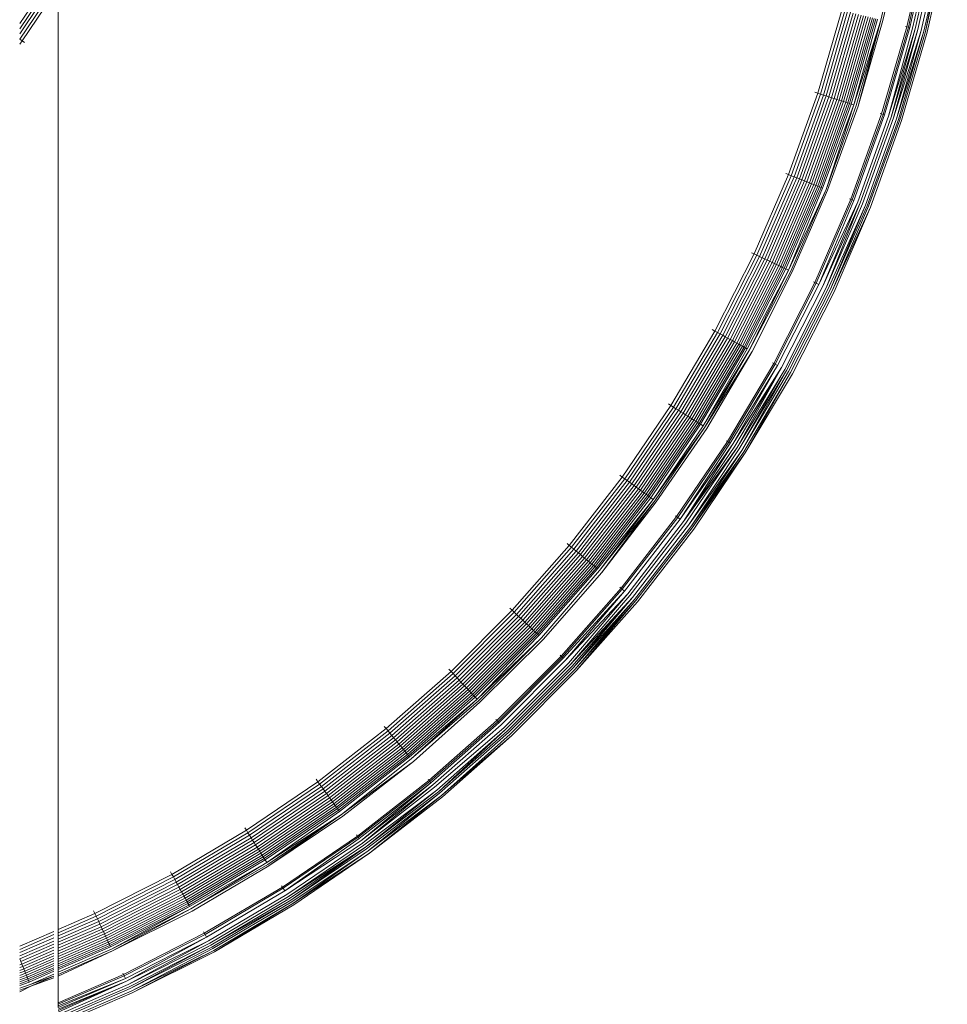
# Model space of a CAD drawing. Units: inches. Extents: x 64 to 1167, y 117 to 939.
# Tile 48 of 56: x 1130.6487 to 1131.3636, y 499.9133 to 500.6716. Entities that reach past the tile are written whole.
import ezdxf

# ---------------------------------------------------------------- set-up
doc = ezdxf.new("R2010")
doc.units = ezdxf.units.IN
doc.header["$MEASUREMENT"] = 0
doc.layers.add('A-FLOR-FIXT', color=8, linetype='Continuous', lineweight=18)

msp = doc.modelspace()

# ---------------------------------------------------------------- linework, layer by layer
at = {"layer": 'A-FLOR-FIXT'}
for p, q in [((1131.3125, 500.67123), (1131.32746, 500.73815)), ((1131.31402, 500.67084), (1131.329, 500.73786)), ((1131.33251, 500.66609), (1131.34775, 500.73428)), ((1131.33362, 500.6658), (1131.34888, 500.73407)), ((1131.33472, 500.66552), (1131.35, 500.73385)), ((1131.33688, 500.66497), (1131.35219, 500.73344)), ((1131.33895, 500.66444), (1131.35428, 500.73304)), ((1131.34088, 500.66394), (1131.35625, 500.73266)), ((1131.34347, 500.66327), (1131.35887, 500.73216)), ((1131.3456, 500.66273), (1131.36103, 500.73175)), ((1131.34672, 500.66244), (1131.36103, 500.73175)), ((1131.34672, 500.66244), (1131.36216, 500.73153)), ((1131.34815, 500.66207), (1131.36362, 500.73126)), ((1130.67845, 500.69852), (1130.67845, 499.97088)), ((1130.64872, 500.66854), (1130.66031, 500.68559)), ((1130.64872, 500.66461), (1130.66217, 500.6844)), ((1130.64872, 500.66061), (1130.66407, 500.6832)), ((1130.64881, 500.6567), (1130.666, 500.68198)), ((1130.65067, 500.65534), (1130.66794, 500.68075)), ((1131.26378, 500.61498), (1131.28237, 500.67896)), ((1131.26596, 500.61427), (1131.28459, 500.67839)), ((1131.26813, 500.61357), (1131.2868, 500.67783)), ((1131.27027, 500.61288), (1131.28898, 500.67727)), ((1131.27237, 500.61219), (1131.29112, 500.67672)), ((1131.27443, 500.61152), (1131.29321, 500.67618)), ((1131.27643, 500.61087), (1131.29525, 500.67566)), ((1131.27837, 500.61024), (1131.29722, 500.67515)), ((1131.28023, 500.60964), (1131.29912, 500.67466)), ((1131.28202, 500.60906), (1131.30094, 500.67419)), ((1131.28371, 500.60851), (1131.30267, 500.67375)), ((1131.28532, 500.60799), (1131.3043, 500.67333)), ((1131.28682, 500.6075), (1131.30583, 500.67294)), ((1131.28821, 500.60705), (1131.30725, 500.67257)), ((1131.28949, 500.60663), (1131.30855, 500.67224)), ((1131.29169, 500.60592), (1131.30973, 500.67194)), ((1131.29169, 500.60592), (1131.3125, 500.67123)), ((1131.29337, 500.60537), (1131.3125, 500.67123)), ((1131.29486, 500.60489), (1131.3125, 500.67123)), ((1131.29486, 500.60489), (1131.31402, 500.67084)), ((1131.31301, 500.59899), (1131.33251, 500.66609)), ((1131.3141, 500.59863), (1131.33362, 500.6658)), ((1131.31519, 500.59828), (1131.33472, 500.66552)), ((1131.33139, 500.66638), (1131.33251, 500.66609)), ((1131.33251, 500.66609), (1131.33362, 500.6658)), ((1131.33362, 500.6658), (1131.33472, 500.66552)), ((1131.31834, 500.59726), (1131.33688, 500.66497)), ((1131.31834, 500.59726), (1131.33895, 500.66444)), ((1131.32031, 500.59662), (1131.33895, 500.66444)), ((1131.32031, 500.59662), (1131.34088, 500.66394)), ((1131.32213, 500.59602), (1131.34088, 500.66394)), ((1131.32213, 500.59602), (1131.34347, 500.66327)), ((1131.32453, 500.59524), (1131.34347, 500.66327)), ((1131.32453, 500.59524), (1131.3456, 500.66273)), ((1131.32587, 500.59481), (1131.3456, 500.66273)), ((1131.32697, 500.59445), (1131.34672, 500.66244)), ((1131.32837, 500.594), (1131.34815, 500.66207)), ((1130.64872, 500.65283), (1130.65067, 500.65534)), ((1130.65067, 500.65534), (1130.64881, 500.6567)), ((1130.65254, 500.65399), (1130.65067, 500.65534)), ((1131.24121, 500.5523), (1131.26378, 500.61498)), ((1131.24335, 500.55145), (1131.26596, 500.61427)), ((1131.24547, 500.55061), (1131.26813, 500.61357)), ((1131.24756, 500.54979), (1131.27027, 500.61288)), ((1131.24961, 500.54897), (1131.27237, 500.61219)), ((1131.26158, 500.6157), (1131.26378, 500.61498)), ((1131.26378, 500.61498), (1131.26596, 500.61427)), ((1131.26596, 500.61427), (1131.26813, 500.61357)), ((1131.26813, 500.61357), (1131.27027, 500.61288)), ((1131.27027, 500.61288), (1131.27237, 500.61219)), ((1131.27237, 500.61219), (1131.27443, 500.61152)), ((1131.25162, 500.54818), (1131.27443, 500.61152)), ((1131.25358, 500.5474), (1131.27643, 500.61087)), ((1131.25547, 500.54665), (1131.27837, 500.61024)), ((1131.25729, 500.54593), (1131.28023, 500.60964)), ((1131.25904, 500.54524), (1131.28202, 500.60906)), ((1131.2607, 500.54458), (1131.28371, 500.60851)), ((1131.26227, 500.54396), (1131.28532, 500.60799)), ((1131.26374, 500.54338), (1131.28682, 500.6075)), ((1131.2651, 500.54284), (1131.28821, 500.60705)), ((1131.26635, 500.54235), (1131.28949, 500.60663)), ((1131.26748, 500.5419), (1131.29169, 500.60592)), ((1131.27014, 500.54085), (1131.29169, 500.60592)), ((1131.27014, 500.54085), (1131.29337, 500.60537)), ((1131.27125, 500.54041), (1131.29486, 500.60489)), ((1131.27443, 500.61152), (1131.27643, 500.61087)), ((1131.27643, 500.61087), (1131.27837, 500.61024)), ((1131.27837, 500.61024), (1131.28023, 500.60964)), ((1131.28023, 500.60964), (1131.28202, 500.60906)), ((1131.28202, 500.60906), (1131.28371, 500.60851)), ((1131.28371, 500.60851), (1131.28532, 500.60799)), ((1131.28532, 500.60799), (1131.28682, 500.6075)), ((1131.28682, 500.6075), (1131.28821, 500.60705)), ((1131.28821, 500.60705), (1131.28949, 500.60663)), ((1131.28949, 500.60663), (1131.29169, 500.60592)), ((1131.28934, 500.53324), (1131.31301, 500.59899)), ((1131.29041, 500.53282), (1131.3141, 500.59863)), ((1131.29147, 500.5324), (1131.31519, 500.59828)), ((1131.29455, 500.53118), (1131.31834, 500.59726)), ((1131.31301, 500.59899), (1131.31191, 500.59934)), ((1131.3141, 500.59863), (1131.31301, 500.59899)), ((1131.31519, 500.59828), (1131.3141, 500.59863)), ((1131.29647, 500.53042), (1131.32031, 500.59662)), ((1131.29826, 500.52971), (1131.32213, 500.59602)), ((1131.3006, 500.52878), (1131.32453, 500.59524)), ((1131.30191, 500.52827), (1131.32587, 500.59481)), ((1131.30298, 500.52784), (1131.32697, 500.59445)), ((1131.30436, 500.5273), (1131.32837, 500.594)), ((1131.21475, 500.49115), (1131.24121, 500.5523)), ((1131.21683, 500.49018), (1131.24335, 500.55145)), ((1131.23906, 500.55315), (1131.24121, 500.5523)), ((1131.24121, 500.5523), (1131.24335, 500.55145)), ((1131.24335, 500.55145), (1131.24547, 500.55061)), ((1131.21889, 500.48921), (1131.24547, 500.55061)), ((1131.22093, 500.48825), (1131.24756, 500.54979)), ((1131.22293, 500.48731), (1131.24961, 500.54897)), ((1131.22488, 500.48639), (1131.25162, 500.54818)), ((1131.22679, 500.48549), (1131.25358, 500.5474)), ((1131.22863, 500.48462), (1131.25547, 500.54665)), ((1131.2304, 500.48379), (1131.25729, 500.54593)), ((1131.2321, 500.48299), (1131.25904, 500.54524)), ((1131.23372, 500.48223), (1131.2607, 500.54458)), ((1131.23524, 500.48151), (1131.26227, 500.54396)), ((1131.24547, 500.55061), (1131.24756, 500.54979)), ((1131.24756, 500.54979), (1131.24961, 500.54897)), ((1131.24961, 500.54897), (1131.25162, 500.54818)), ((1131.25162, 500.54818), (1131.25358, 500.5474)), ((1131.25358, 500.5474), (1131.25547, 500.54665)), ((1131.25547, 500.54665), (1131.25729, 500.54593)), ((1131.25729, 500.54593), (1131.25904, 500.54524)), ((1131.25904, 500.54524), (1131.2607, 500.54458)), ((1131.2607, 500.54458), (1131.26227, 500.54396)), ((1131.26227, 500.54396), (1131.26374, 500.54338)), ((1131.23667, 500.48084), (1131.26374, 500.54338)), ((1131.238, 500.48022), (1131.2651, 500.54284)), ((1131.23921, 500.47964), (1131.26635, 500.54235)), ((1131.2413, 500.47866), (1131.26748, 500.5419)), ((1131.2413, 500.47866), (1131.27014, 500.54085)), ((1131.2429, 500.47791), (1131.27014, 500.54085)), ((1131.24398, 500.4774), (1131.27125, 500.54041)), ((1131.26374, 500.54338), (1131.2651, 500.54284)), ((1131.2651, 500.54284), (1131.26635, 500.54235)), ((1131.26635, 500.54235), (1131.26748, 500.5419)), ((1131.26159, 500.46911), (1131.28934, 500.53324)), ((1131.26263, 500.46862), (1131.29041, 500.53282)), ((1131.26468, 500.46766), (1131.29147, 500.5324)), ((1131.26468, 500.46766), (1131.29455, 500.53118)), ((1131.26761, 500.46628), (1131.29455, 500.53118)), ((1131.26761, 500.46628), (1131.29647, 500.53042)), ((1131.27027, 500.46503), (1131.29647, 500.53042)), ((1131.27027, 500.46503), (1131.29826, 500.52971)), ((1131.27184, 500.46429), (1131.3006, 500.52878)), ((1131.27321, 500.46364), (1131.3006, 500.52878)), ((1131.28827, 500.53367), (1131.28934, 500.53324)), ((1131.28934, 500.53324), (1131.29041, 500.53282)), ((1131.29041, 500.53282), (1131.29147, 500.5324)), ((1131.27321, 500.46364), (1131.30191, 500.52827)), ((1131.27487, 500.46287), (1131.30298, 500.52784)), ((1131.27487, 500.46287), (1131.30436, 500.5273)), ((1131.27651, 500.46209), (1131.30436, 500.5273)), ((1131.1845, 500.43179), (1131.21475, 500.49115)), ((1131.21266, 500.49214), (1131.21475, 500.49115)), ((1131.21475, 500.49115), (1131.21683, 500.49018)), ((1131.18652, 500.43068), (1131.21683, 500.49018)), ((1131.18851, 500.42959), (1131.21889, 500.48921)), ((1131.19049, 500.4285), (1131.22093, 500.48825)), ((1131.19242, 500.42744), (1131.22293, 500.48731)), ((1131.19432, 500.4264), (1131.22488, 500.48639)), ((1131.19616, 500.42538), (1131.22679, 500.48549)), ((1131.19794, 500.4244), (1131.22863, 500.48462)), ((1131.19966, 500.42346), (1131.2304, 500.48379)), ((1131.21683, 500.49018), (1131.21889, 500.48921)), ((1131.21889, 500.48921), (1131.22093, 500.48825)), ((1131.22093, 500.48825), (1131.22293, 500.48731)), ((1131.22293, 500.48731), (1131.22488, 500.48639)), ((1131.22488, 500.48639), (1131.22679, 500.48549)), ((1131.22679, 500.48549), (1131.22863, 500.48462)), ((1131.22863, 500.48462), (1131.2304, 500.48379)), ((1131.2304, 500.48379), (1131.2321, 500.48299)), ((1131.20131, 500.42255), (1131.2321, 500.48299)), ((1131.20287, 500.42169), (1131.23372, 500.48223)), ((1131.20435, 500.42088), (1131.23524, 500.48151)), ((1131.20573, 500.42012), (1131.23667, 500.48084)), ((1131.20702, 500.41941), (1131.238, 500.48022)), ((1131.2082, 500.41877), (1131.23921, 500.47964)), ((1131.20926, 500.41818), (1131.2413, 500.47866)), ((1131.21105, 500.4172), (1131.2413, 500.47866)), ((1131.21105, 500.4172), (1131.2429, 500.47791)), ((1131.21334, 500.41594), (1131.24398, 500.4774)), ((1131.2321, 500.48299), (1131.23372, 500.48223)), ((1131.23372, 500.48223), (1131.23524, 500.48151)), ((1131.23524, 500.48151), (1131.23667, 500.48084)), ((1131.23667, 500.48084), (1131.238, 500.48022)), ((1131.238, 500.48022), (1131.23921, 500.47964)), ((1131.23921, 500.47964), (1131.2413, 500.47866)), ((1131.22987, 500.40685), (1131.26159, 500.46911)), ((1131.23087, 500.4063), (1131.26263, 500.46862)), ((1131.26055, 500.4696), (1131.26159, 500.46911)), ((1131.26159, 500.46911), (1131.26263, 500.46862)), ((1131.26263, 500.46862), (1131.26468, 500.46766)), ((1131.23286, 500.40521), (1131.26468, 500.46766)), ((1131.2357, 500.40365), (1131.26761, 500.46628)), ((1131.23827, 500.40223), (1131.27027, 500.46503)), ((1131.23979, 500.4014), (1131.27184, 500.46429)), ((1131.24112, 500.40066), (1131.27321, 500.46364)), ((1131.24272, 500.39978), (1131.27487, 500.46287)), ((1131.24432, 500.39891), (1131.27651, 500.46209)), ((1131.15059, 500.37445), (1131.1845, 500.43179)), ((1131.15253, 500.37321), (1131.18652, 500.43068)), ((1131.1845, 500.43179), (1131.18248, 500.4329)), ((1131.18652, 500.43068), (1131.1845, 500.43179)), ((1131.18851, 500.42959), (1131.18652, 500.43068)), ((1131.15445, 500.37199), (1131.18851, 500.42959)), ((1131.15635, 500.37079), (1131.19049, 500.4285)), ((1131.15822, 500.3696), (1131.19242, 500.42744)), ((1131.16004, 500.36845), (1131.19432, 500.4264)), ((1131.16182, 500.36732), (1131.19616, 500.42538)), ((1131.16354, 500.36623), (1131.19794, 500.4244)), ((1131.1652, 500.36518), (1131.19966, 500.42346)), ((1131.16678, 500.36417), (1131.20131, 500.42255)), ((1131.19049, 500.4285), (1131.18851, 500.42959)), ((1131.19242, 500.42744), (1131.19049, 500.4285)), ((1131.19432, 500.4264), (1131.19242, 500.42744)), ((1131.19616, 500.42538), (1131.19432, 500.4264)), ((1131.19794, 500.4244), (1131.19616, 500.42538)), ((1131.19966, 500.42346), (1131.19794, 500.4244)), ((1131.20131, 500.42255), (1131.19966, 500.42346)), ((1131.20287, 500.42169), (1131.20131, 500.42255)), ((1131.16829, 500.36321), (1131.20287, 500.42169)), ((1131.16971, 500.36231), (1131.20435, 500.42088)), ((1131.17104, 500.36146), (1131.20573, 500.42012)), ((1131.17228, 500.36068), (1131.20702, 500.41941)), ((1131.17342, 500.35996), (1131.2082, 500.41877)), ((1131.17537, 500.35872), (1131.20926, 500.41818)), ((1131.17537, 500.35872), (1131.21105, 500.4172)), ((1131.17686, 500.35778), (1131.21105, 500.4172)), ((1131.17686, 500.35778), (1131.21334, 500.41594)), ((1131.17837, 500.35681), (1131.21334, 500.41594)), ((1131.20435, 500.42088), (1131.20287, 500.42169)), ((1131.20573, 500.42012), (1131.20435, 500.42088)), ((1131.20702, 500.41941), (1131.20573, 500.42012)), ((1131.2082, 500.41877), (1131.20702, 500.41941)), ((1131.20926, 500.41818), (1131.2082, 500.41877)), ((1131.22987, 500.40685), (1131.22886, 500.40741)), ((1131.1943, 500.34671), (1131.22987, 500.40685)), ((1131.19527, 500.34609), (1131.23087, 500.4063)), ((1131.19623, 500.34548), (1131.23286, 500.40521)), ((1131.19811, 500.34429), (1131.23286, 500.40521)), ((1131.19811, 500.34429), (1131.2357, 500.40365)), ((1131.19991, 500.34314), (1131.2357, 500.40365)), ((1131.2016, 500.34207), (1131.2357, 500.40365)), ((1131.2016, 500.34207), (1131.23827, 500.40223)), ((1131.20315, 500.34109), (1131.23827, 500.40223)), ((1131.20315, 500.34109), (1131.23979, 500.4014)), ((1131.20514, 500.33982), (1131.23979, 500.4014)), ((1131.20514, 500.33982), (1131.24112, 500.40066)), ((1131.20669, 500.33885), (1131.24272, 500.39978)), ((1131.20794, 500.33805), (1131.24272, 500.39978)), ((1131.23087, 500.4063), (1131.22987, 500.40685)), ((1131.23286, 500.40521), (1131.23087, 500.4063)), ((1131.20794, 500.33805), (1131.24432, 500.39891)), ((1131.11314, 500.31934), (1131.15059, 500.37445)), ((1131.115, 500.31799), (1131.15253, 500.37321)), ((1131.11684, 500.31665), (1131.15445, 500.37199)), ((1131.11866, 500.31533), (1131.15635, 500.37079)), ((1131.12045, 500.31403), (1131.15822, 500.3696)), ((1131.14864, 500.37568), (1131.15059, 500.37445)), ((1131.15059, 500.37445), (1131.15253, 500.37321)), ((1131.15253, 500.37321), (1131.15445, 500.37199)), ((1131.15445, 500.37199), (1131.15635, 500.37079)), ((1131.15635, 500.37079), (1131.15822, 500.3696)), ((1131.15822, 500.3696), (1131.16004, 500.36845)), ((1131.1222, 500.31276), (1131.16004, 500.36845)), ((1131.1239, 500.31152), (1131.16182, 500.36732)), ((1131.12555, 500.31033), (1131.16354, 500.36623)), ((1131.12714, 500.30917), (1131.1652, 500.36518)), ((1131.12865, 500.30807), (1131.16678, 500.36417)), ((1131.1301, 500.30702), (1131.16829, 500.36321)), ((1131.13146, 500.30603), (1131.16971, 500.36231)), ((1131.16004, 500.36845), (1131.16182, 500.36732)), ((1131.16182, 500.36732), (1131.16354, 500.36623)), ((1131.16354, 500.36623), (1131.1652, 500.36518)), ((1131.1652, 500.36518), (1131.16678, 500.36417)), ((1131.16678, 500.36417), (1131.16829, 500.36321)), ((1131.16829, 500.36321), (1131.16971, 500.36231)), ((1131.16971, 500.36231), (1131.17104, 500.36146)), ((1131.13274, 500.3051), (1131.17104, 500.36146)), ((1131.13393, 500.30424), (1131.17228, 500.36068)), ((1131.13501, 500.30345), (1131.17342, 500.35996)), ((1131.13688, 500.30209), (1131.17537, 500.35872)), ((1131.13688, 500.30209), (1131.17686, 500.35778)), ((1131.13831, 500.30105), (1131.17686, 500.35778)), ((1131.13928, 500.30035), (1131.17837, 500.35681)), ((1131.17104, 500.36146), (1131.17228, 500.36068)), ((1131.17228, 500.36068), (1131.17342, 500.35996)), ((1131.17342, 500.35996), (1131.17537, 500.35872)), ((1131.15502, 500.28891), (1131.1943, 500.34671)), ((1131.19332, 500.34733), (1131.1943, 500.34671)), ((1131.1943, 500.34671), (1131.19527, 500.34609)), ((1131.15595, 500.28824), (1131.19527, 500.34609)), ((1131.15778, 500.28691), (1131.19623, 500.34548)), ((1131.15778, 500.28691), (1131.19811, 500.34429)), ((1131.1604, 500.285), (1131.19811, 500.34429)), ((1131.1604, 500.285), (1131.19991, 500.34314)), ((1131.1604, 500.285), (1131.2016, 500.34207)), ((1131.16202, 500.28383), (1131.2016, 500.34207)), ((1131.16418, 500.28226), (1131.20315, 500.34109)), ((1131.16418, 500.28226), (1131.20514, 500.33982)), ((1131.16596, 500.28097), (1131.20514, 500.33982)), ((1131.19527, 500.34609), (1131.19623, 500.34548)), ((1131.16596, 500.28097), (1131.20669, 500.33885)), ((1131.16689, 500.28029), (1131.20669, 500.33885)), ((1131.16689, 500.28029), (1131.20794, 500.33805)), ((1131.16824, 500.27931), (1131.20794, 500.33805)), ((1131.07231, 500.2667), (1131.11314, 500.31934)), ((1131.07408, 500.26523), (1131.115, 500.31799)), ((1131.07583, 500.26378), (1131.11684, 500.31665)), ((1131.11127, 500.3207), (1131.11314, 500.31934)), ((1131.11314, 500.31934), (1131.115, 500.31799)), ((1131.115, 500.31799), (1131.11684, 500.31665)), ((1131.11684, 500.31665), (1131.11866, 500.31533)), ((1131.07757, 500.26235), (1131.11866, 500.31533)), ((1131.07927, 500.26094), (1131.12045, 500.31403)), ((1131.08093, 500.25956), (1131.1222, 500.31276)), ((1131.08256, 500.25822), (1131.1239, 500.31152)), ((1131.08412, 500.25692), (1131.12555, 500.31033)), ((1131.08564, 500.25567), (1131.12714, 500.30917)), ((1131.11866, 500.31533), (1131.12045, 500.31403)), ((1131.12045, 500.31403), (1131.1222, 500.31276)), ((1131.1222, 500.31276), (1131.1239, 500.31152)), ((1131.1239, 500.31152), (1131.12555, 500.31033)), ((1131.12555, 500.31033), (1131.12714, 500.30917)), ((1131.12714, 500.30917), (1131.12865, 500.30807)), ((1131.08708, 500.25447), (1131.12865, 500.30807)), ((1131.08846, 500.25334), (1131.1301, 500.30702)), ((1131.08976, 500.25226), (1131.13146, 500.30603)), ((1131.09097, 500.25126), (1131.13274, 500.3051)), ((1131.0921, 500.25032), (1131.13393, 500.30424)), ((1131.09314, 500.24946), (1131.13501, 500.30345)), ((1131.09408, 500.24869), (1131.13688, 500.30209)), ((1131.09565, 500.24739), (1131.13688, 500.30209)), ((1131.12865, 500.30807), (1131.1301, 500.30702)), ((1131.1301, 500.30702), (1131.13146, 500.30603)), ((1131.13146, 500.30603), (1131.13274, 500.3051)), ((1131.13274, 500.3051), (1131.13393, 500.30424)), ((1131.13393, 500.30424), (1131.13501, 500.30345)), ((1131.13501, 500.30345), (1131.13688, 500.30209)), ((1131.09565, 500.24739), (1131.13831, 500.30105)), ((1131.09749, 500.24587), (1131.13831, 500.30105)), ((1131.09749, 500.24587), (1131.13928, 500.30035)), ((1131.11219, 500.2337), (1131.15502, 500.28891)), ((1131.11308, 500.23297), (1131.15595, 500.28824)), ((1131.11482, 500.23152), (1131.15778, 500.28691)), ((1131.15502, 500.28891), (1131.15409, 500.28959)), ((1131.15595, 500.28824), (1131.15502, 500.28891)), ((1131.15778, 500.28691), (1131.15595, 500.28824)), ((1131.11732, 500.22946), (1131.1604, 500.285)), ((1131.11886, 500.22819), (1131.16202, 500.28383)), ((1131.12092, 500.22648), (1131.16418, 500.28226)), ((1131.12261, 500.22508), (1131.16596, 500.28097)), ((1131.1235, 500.22435), (1131.16689, 500.28029)), ((1131.12478, 500.22328), (1131.16824, 500.27931)), ((1131.02825, 500.21672), (1131.07231, 500.2667)), ((1131.02992, 500.21515), (1131.07408, 500.26523)), ((1131.03158, 500.21359), (1131.07583, 500.26378)), ((1131.07053, 500.26817), (1131.07231, 500.2667)), ((1131.07231, 500.2667), (1131.07408, 500.26523)), ((1131.07408, 500.26523), (1131.07583, 500.26378)), ((1131.07583, 500.26378), (1131.07757, 500.26235)), ((1131.03322, 500.21205), (1131.07757, 500.26235)), ((1131.03483, 500.21054), (1131.07927, 500.26094)), ((1131.03641, 500.20906), (1131.08093, 500.25956)), ((1131.03794, 500.20762), (1131.08256, 500.25822)), ((1131.03943, 500.20622), (1131.08412, 500.25692)), ((1131.07757, 500.26235), (1131.07927, 500.26094)), ((1131.07927, 500.26094), (1131.08093, 500.25956)), ((1131.08093, 500.25956), (1131.08256, 500.25822)), ((1131.08256, 500.25822), (1131.08412, 500.25692)), ((1131.08412, 500.25692), (1131.08564, 500.25567)), ((1131.04086, 500.20488), (1131.08564, 500.25567)), ((1131.04223, 500.2036), (1131.08708, 500.25447)), ((1131.04353, 500.20237), (1131.08846, 500.25334)), ((1131.04476, 500.20122), (1131.08976, 500.25226)), ((1131.04591, 500.20014), (1131.09097, 500.25126)), ((1131.04697, 500.19914), (1131.0921, 500.25032)), ((1131.04796, 500.19821), (1131.09314, 500.24946)), ((1131.04884, 500.19738), (1131.09408, 500.24869)), ((1131.08564, 500.25567), (1131.08708, 500.25447)), ((1131.08708, 500.25447), (1131.08846, 500.25334)), ((1131.08846, 500.25334), (1131.08976, 500.25226)), ((1131.08976, 500.25226), (1131.09097, 500.25126)), ((1131.09097, 500.25126), (1131.0921, 500.25032)), ((1131.0921, 500.25032), (1131.09314, 500.24946)), ((1131.09314, 500.24946), (1131.09408, 500.24869)), ((1131.05093, 500.19543), (1131.09565, 500.24739)), ((1131.05224, 500.19419), (1131.09749, 500.24587)), ((1131.06598, 500.18129), (1131.11219, 500.2337)), ((1131.06682, 500.1805), (1131.11308, 500.23297)), ((1131.11219, 500.2337), (1131.1113, 500.23444)), ((1131.11308, 500.23297), (1131.11219, 500.2337)), ((1131.11482, 500.23152), (1131.11308, 500.23297)), ((1131.06765, 500.17972), (1131.11482, 500.23152)), ((1131.06928, 500.17819), (1131.11482, 500.23152)), ((1131.06928, 500.17819), (1131.11732, 500.22946)), ((1131.07157, 500.17604), (1131.11732, 500.22946)), ((1131.07297, 500.17472), (1131.11886, 500.22819)), ((1131.07297, 500.17472), (1131.12092, 500.22648)), ((1131.07424, 500.17353), (1131.12092, 500.22648)), ((1131.07535, 500.17249), (1131.12092, 500.22648)), ((1131.02656, 500.2183), (1131.02825, 500.21672)), ((1131.07535, 500.17249), (1131.12261, 500.22508)), ((1131.07668, 500.17124), (1131.12261, 500.22508)), ((1131.07668, 500.17124), (1131.1235, 500.22435)), ((1131.07776, 500.17023), (1131.1235, 500.22435)), ((1131.07776, 500.17023), (1131.12478, 500.22328)), ((1130.98114, 500.16961), (1131.02825, 500.21672)), ((1130.98271, 500.16794), (1131.02992, 500.21515)), ((1130.98427, 500.16628), (1131.03158, 500.21359)), ((1130.98581, 500.16464), (1131.03322, 500.21205)), ((1130.98732, 500.16302), (1131.03483, 500.21054)), ((1131.02825, 500.21672), (1131.02992, 500.21515)), ((1131.02992, 500.21515), (1131.03158, 500.21359)), ((1131.03158, 500.21359), (1131.03322, 500.21205)), ((1131.03322, 500.21205), (1131.03483, 500.21054)), ((1131.03483, 500.21054), (1131.03641, 500.20906)), ((1130.9888, 500.16145), (1131.03641, 500.20906)), ((1130.99024, 500.15992), (1131.03794, 500.20762)), ((1130.99164, 500.15843), (1131.03943, 500.20622)), ((1130.99298, 500.157), (1131.04086, 500.20488)), ((1130.99426, 500.15563), (1131.04223, 500.2036)), ((1131.03641, 500.20906), (1131.03794, 500.20762)), ((1131.03794, 500.20762), (1131.03943, 500.20622)), ((1131.03943, 500.20622), (1131.04086, 500.20488)), ((1131.04086, 500.20488), (1131.04223, 500.2036)), ((1131.04223, 500.2036), (1131.04353, 500.20237)), ((1130.99549, 500.15433), (1131.04353, 500.20237)), ((1130.99664, 500.1531), (1131.04476, 500.20122)), ((1130.99772, 500.15195), (1131.04591, 500.20014)), ((1130.99872, 500.15088), (1131.04697, 500.19914)), ((1130.99964, 500.1499), (1131.04796, 500.19821)), ((1131.00122, 500.14822), (1131.04884, 500.19738)), ((1131.00122, 500.14822), (1131.05093, 500.19543)), ((1131.00243, 500.14693), (1131.05093, 500.19543)), ((1131.04353, 500.20237), (1131.04476, 500.20122)), ((1131.04476, 500.20122), (1131.04591, 500.20014)), ((1131.04591, 500.20014), (1131.04697, 500.19914)), ((1131.04697, 500.19914), (1131.04796, 500.19821)), ((1131.04796, 500.19821), (1131.04884, 500.19738)), ((1131.00325, 500.14606), (1131.05224, 500.19419)), ((1131.01657, 500.13188), (1131.06598, 500.18129)), ((1131.01736, 500.13104), (1131.06682, 500.1805)), ((1131.06514, 500.18208), (1131.06598, 500.18129)), ((1131.06598, 500.18129), (1131.06682, 500.1805)), ((1131.06682, 500.1805), (1131.06765, 500.17972)), ((1131.01814, 500.13021), (1131.06765, 500.17972)), ((1131.01967, 500.12858), (1131.06928, 500.17819)), ((1131.02182, 500.12628), (1131.07157, 500.17604)), ((1131.02314, 500.12489), (1131.07297, 500.17472)), ((1131.02432, 500.12362), (1131.07424, 500.17353)), ((1131.02537, 500.12251), (1131.07535, 500.17249)), ((1130.93116, 500.12555), (1130.98114, 500.16961)), ((1130.93263, 500.12378), (1130.98271, 500.16794)), ((1130.93408, 500.12203), (1130.98427, 500.16628)), ((1130.97956, 500.17129), (1130.98114, 500.16961)), ((1130.98114, 500.16961), (1130.98271, 500.16794)), ((1130.98271, 500.16794), (1130.98427, 500.16628)), ((1130.98427, 500.16628), (1130.98581, 500.16464)), ((1131.02662, 500.12118), (1131.07668, 500.17124)), ((1131.02763, 500.1201), (1131.07776, 500.17023)), ((1130.93551, 500.12029), (1130.98581, 500.16464)), ((1130.93692, 500.11859), (1130.98732, 500.16302)), ((1130.9383, 500.11692), (1130.9888, 500.16145)), ((1130.93964, 500.1153), (1130.99024, 500.15992)), ((1130.94094, 500.11373), (1130.99164, 500.15843)), ((1130.98581, 500.16464), (1130.98732, 500.16302)), ((1130.98732, 500.16302), (1130.9888, 500.16145)), ((1130.9888, 500.16145), (1130.99024, 500.15992)), ((1130.99024, 500.15992), (1130.99164, 500.15843)), ((1130.99164, 500.15843), (1130.99298, 500.157)), ((1130.94219, 500.11222), (1130.99298, 500.157)), ((1130.94338, 500.11078), (1130.99426, 500.15563)), ((1130.94452, 500.1094), (1130.99549, 500.15433)), ((1130.9456, 500.1081), (1130.99664, 500.1531)), ((1130.9466, 500.10689), (1130.99772, 500.15195)), ((1130.94754, 500.10576), (1130.99872, 500.15088)), ((1130.94839, 500.10472), (1130.99964, 500.1499)), ((1130.99298, 500.157), (1130.99426, 500.15563)), ((1130.99426, 500.15563), (1130.99549, 500.15433)), ((1130.99549, 500.15433), (1130.99664, 500.1531)), ((1130.99664, 500.1531), (1130.99772, 500.15195)), ((1130.99772, 500.15195), (1130.99872, 500.15088)), ((1130.99872, 500.15088), (1130.99964, 500.1499)), ((1130.99964, 500.1499), (1131.00122, 500.14822)), ((1130.94917, 500.10378), (1131.00122, 500.14822)), ((1130.95047, 500.10221), (1131.00122, 500.14822)), ((1130.95047, 500.10221), (1131.00243, 500.14693)), ((1130.95214, 500.1002), (1131.00325, 500.14606)), ((1130.92969, 500.12733), (1130.93116, 500.12555)), ((1130.96416, 500.08567), (1131.01657, 500.13188)), ((1130.96489, 500.08478), (1131.01736, 500.13104)), ((1130.96562, 500.0839), (1131.01814, 500.13021)), ((1130.96704, 500.08218), (1131.01967, 500.12858)), ((1131.01578, 500.13272), (1131.01657, 500.13188)), ((1131.01657, 500.13188), (1131.01736, 500.13104)), ((1131.01736, 500.13104), (1131.01814, 500.13021)), ((1130.87852, 500.08472), (1130.93116, 500.12555)), ((1130.87987, 500.08286), (1130.93263, 500.12378)), ((1130.88121, 500.08101), (1130.93408, 500.12203)), ((1130.88253, 500.0792), (1130.93551, 500.12029)), ((1130.93116, 500.12555), (1130.93263, 500.12378)), ((1130.93263, 500.12378), (1130.93408, 500.12203)), ((1130.93408, 500.12203), (1130.93551, 500.12029)), ((1130.93551, 500.12029), (1130.93692, 500.11859)), ((1130.9684, 500.08054), (1131.02182, 500.12628)), ((1130.97027, 500.07828), (1131.02314, 500.12489)), ((1130.97138, 500.07694), (1131.02314, 500.12489)), ((1130.97138, 500.07694), (1131.02432, 500.12362)), ((1130.97235, 500.07577), (1131.02537, 500.12251)), ((1130.97381, 500.07399), (1131.02662, 500.12118)), ((1130.97381, 500.07399), (1131.02763, 500.1201)), ((1130.97465, 500.07299), (1131.02763, 500.1201)), ((1130.88383, 500.07741), (1130.93692, 500.11859)), ((1130.8851, 500.07566), (1130.9383, 500.11692)), ((1130.88634, 500.07396), (1130.93964, 500.1153)), ((1130.88753, 500.07231), (1130.94094, 500.11373)), ((1130.88869, 500.07072), (1130.94219, 500.11222)), ((1130.93692, 500.11859), (1130.9383, 500.11692)), ((1130.9383, 500.11692), (1130.93964, 500.1153)), ((1130.93964, 500.1153), (1130.94094, 500.11373)), ((1130.94094, 500.11373), (1130.94219, 500.11222)), ((1130.94219, 500.11222), (1130.94338, 500.11078)), ((1130.88979, 500.0692), (1130.94338, 500.11078)), ((1130.89084, 500.06776), (1130.94452, 500.1094)), ((1130.89183, 500.0664), (1130.9456, 500.1081)), ((1130.89276, 500.06512), (1130.9466, 500.10689)), ((1130.89362, 500.06393), (1130.94754, 500.10576)), ((1130.89441, 500.06284), (1130.94839, 500.10472)), ((1130.94338, 500.11078), (1130.94452, 500.1094)), ((1130.94452, 500.1094), (1130.9456, 500.1081)), ((1130.9456, 500.1081), (1130.9466, 500.10689)), ((1130.9466, 500.10689), (1130.94754, 500.10576)), ((1130.94754, 500.10576), (1130.94839, 500.10472)), ((1130.94839, 500.10472), (1130.94917, 500.10378)), ((1130.89513, 500.06186), (1130.94917, 500.10378)), ((1130.8968, 500.05955), (1130.95047, 500.10221)), ((1130.8968, 500.05955), (1130.95214, 500.1002)), ((1130.89786, 500.05809), (1130.95214, 500.1002)), ((1130.82341, 500.04727), (1130.87852, 500.08472)), ((1130.82465, 500.04533), (1130.87987, 500.08286)), ((1130.87852, 500.08472), (1130.87716, 500.08659)), ((1130.87987, 500.08286), (1130.87852, 500.08472)), ((1130.88121, 500.08101), (1130.87987, 500.08286)), ((1130.90894, 500.04284), (1130.96416, 500.08567)), ((1130.90962, 500.04191), (1130.96489, 500.08478)), ((1130.91029, 500.04099), (1130.96562, 500.0839)), ((1130.9116, 500.03918), (1130.96562, 500.0839)), ((1130.9116, 500.03918), (1130.96704, 500.08218)), ((1130.91285, 500.03746), (1130.96704, 500.08218)), ((1130.96342, 500.08655), (1130.96416, 500.08567)), ((1130.96416, 500.08567), (1130.96489, 500.08478)), ((1130.96489, 500.08478), (1130.96562, 500.0839)), ((1130.82587, 500.0434), (1130.88121, 500.08101)), ((1130.82707, 500.04151), (1130.88253, 500.0792)), ((1130.82826, 500.03964), (1130.88383, 500.07741)), ((1130.82941, 500.03781), (1130.8851, 500.07566)), ((1130.83054, 500.03604), (1130.88634, 500.07396)), ((1130.88253, 500.0792), (1130.88121, 500.08101)), ((1130.88383, 500.07741), (1130.88253, 500.0792)), ((1130.8851, 500.07566), (1130.88383, 500.07741)), ((1130.88634, 500.07396), (1130.8851, 500.07566)), ((1130.88753, 500.07231), (1130.88634, 500.07396)), ((1130.91285, 500.03746), (1130.9684, 500.08054)), ((1130.91403, 500.03584), (1130.97027, 500.07828)), ((1130.91511, 500.03436), (1130.97027, 500.07828)), ((1130.91511, 500.03436), (1130.97138, 500.07694)), ((1130.91606, 500.03304), (1130.97235, 500.07577)), ((1130.91725, 500.03141), (1130.97235, 500.07577)), ((1130.91725, 500.03141), (1130.97381, 500.07399)), ((1130.91844, 500.02977), (1130.97381, 500.07399)), ((1130.83163, 500.03432), (1130.88753, 500.07231)), ((1130.83268, 500.03266), (1130.88869, 500.07072)), ((1130.83369, 500.03108), (1130.88979, 500.0692)), ((1130.83465, 500.02957), (1130.89084, 500.06776)), ((1130.83555, 500.02815), (1130.89183, 500.0664)), ((1130.88869, 500.07072), (1130.88753, 500.07231)), ((1130.88979, 500.0692), (1130.88869, 500.07072)), ((1130.89084, 500.06776), (1130.88979, 500.0692)), ((1130.89183, 500.0664), (1130.89084, 500.06776)), ((1130.89276, 500.06512), (1130.89183, 500.0664)), ((1130.91844, 500.02977), (1130.97465, 500.07299)), ((1130.83639, 500.02681), (1130.89276, 500.06512)), ((1130.83718, 500.02558), (1130.89362, 500.06393)), ((1130.8379, 500.02444), (1130.89441, 500.06284)), ((1130.83914, 500.02249), (1130.89513, 500.06186)), ((1130.83914, 500.02249), (1130.8968, 500.05955)), ((1130.84008, 500.021), (1130.8968, 500.05955)), ((1130.84072, 500.01999), (1130.8968, 500.05955)), ((1130.89362, 500.06393), (1130.89276, 500.06512)), ((1130.89441, 500.06284), (1130.89362, 500.06393)), ((1130.89513, 500.06186), (1130.89441, 500.06284)), ((1130.84072, 500.01999), (1130.89786, 500.05809)), ((1130.76607, 500.01335), (1130.82341, 500.04727)), ((1130.76717, 500.01134), (1130.82465, 500.04533)), ((1130.76827, 500.00934), (1130.82587, 500.0434)), ((1130.82218, 500.04922), (1130.82341, 500.04727)), ((1130.82341, 500.04727), (1130.82465, 500.04533)), ((1130.82465, 500.04533), (1130.82587, 500.0434)), ((1130.82587, 500.0434), (1130.82707, 500.04151)), ((1130.90827, 500.04377), (1130.90894, 500.04284)), ((1130.76936, 500.00737), (1130.82707, 500.04151)), ((1130.77042, 500.00544), (1130.82826, 500.03964)), ((1130.77146, 500.00354), (1130.82941, 500.03781)), ((1130.77248, 500.0017), (1130.83054, 500.03604)), ((1130.82707, 500.04151), (1130.82826, 500.03964)), ((1130.82826, 500.03964), (1130.82941, 500.03781)), ((1130.82941, 500.03781), (1130.83054, 500.03604)), ((1130.83054, 500.03604), (1130.83163, 500.03432)), ((1130.85115, 500.00356), (1130.90894, 500.04284)), ((1130.85177, 500.00259), (1130.90962, 500.04191)), ((1130.85298, 500.00068), (1130.91029, 500.04099)), ((1130.85298, 500.00068), (1130.9116, 500.03918)), ((1130.85472, 499.99795), (1130.91285, 500.03746)), ((1130.85579, 499.99626), (1130.91403, 500.03584)), ((1130.90894, 500.04284), (1130.90962, 500.04191)), ((1130.90962, 500.04191), (1130.91029, 500.04099)), ((1130.77346, 499.99991), (1130.83163, 500.03432)), ((1130.7744, 499.9982), (1130.83268, 500.03266)), ((1130.77531, 499.99655), (1130.83369, 500.03108)), ((1130.77617, 499.99499), (1130.83465, 500.02957)), ((1130.83163, 500.03432), (1130.83268, 500.03266)), ((1130.83268, 500.03266), (1130.83369, 500.03108)), ((1130.83369, 500.03108), (1130.83465, 500.02957)), ((1130.83465, 500.02957), (1130.83555, 500.02815)), ((1130.85579, 499.99626), (1130.91511, 500.03436)), ((1130.85677, 499.99471), (1130.91511, 500.03436)), ((1130.85764, 499.99333), (1130.91511, 500.03436)), ((1130.85764, 499.99333), (1130.91606, 500.03304)), ((1130.85839, 499.99215), (1130.91725, 500.03141)), ((1130.85927, 499.99077), (1130.91725, 500.03141)), ((1130.85927, 499.99077), (1130.91844, 500.02977)), ((1130.85991, 499.98976), (1130.91844, 500.02977)), ((1130.77698, 499.99351), (1130.83555, 500.02815)), ((1130.77774, 499.99213), (1130.83639, 500.02681)), ((1130.77844, 499.99084), (1130.83718, 500.02558)), ((1130.77909, 499.98966), (1130.8379, 500.02444)), ((1130.77968, 499.98859), (1130.83914, 500.02249)), ((1130.78066, 499.9868), (1130.83914, 500.02249)), ((1130.78066, 499.9868), (1130.84008, 500.021)), ((1130.83555, 500.02815), (1130.83639, 500.02681)), ((1130.83639, 500.02681), (1130.83718, 500.02558)), ((1130.83718, 500.02558), (1130.8379, 500.02444)), ((1130.8379, 500.02444), (1130.83914, 500.02249)), ((1130.7067, 499.98311), (1130.76607, 500.01335)), ((1130.76607, 500.01335), (1130.76496, 500.01538)), ((1130.76717, 500.01134), (1130.76607, 500.01335)), ((1130.78163, 499.98504), (1130.84072, 500.01999)), ((1130.70768, 499.98103), (1130.76717, 500.01134)), ((1130.70865, 499.97897), (1130.76827, 500.00934)), ((1130.70961, 499.97693), (1130.76936, 500.00737)), ((1130.76827, 500.00934), (1130.76717, 500.01134)), ((1130.76936, 500.00737), (1130.76827, 500.00934)), ((1130.77042, 500.00544), (1130.76936, 500.00737)), ((1130.71055, 499.97493), (1130.77042, 500.00544)), ((1130.71147, 499.97298), (1130.77146, 500.00354)), ((1130.71237, 499.97107), (1130.77248, 500.0017)), ((1130.71323, 499.96923), (1130.77346, 499.99991)), ((1130.71407, 499.96746), (1130.7744, 499.9982)), ((1130.77146, 500.00354), (1130.77042, 500.00544)), ((1130.77248, 500.0017), (1130.77146, 500.00354)), ((1130.77346, 499.99991), (1130.77248, 500.0017)), ((1130.7744, 499.9982), (1130.77346, 499.99991)), ((1130.77531, 499.99655), (1130.7744, 499.9982)), ((1130.79101, 499.96799), (1130.85115, 500.00356)), ((1130.79156, 499.96698), (1130.85177, 500.00259)), ((1130.79265, 499.965), (1130.85298, 500.00068)), ((1130.79421, 499.96216), (1130.85472, 499.99795)), ((1130.85115, 500.00356), (1130.85053, 500.00454)), ((1130.85177, 500.00259), (1130.85115, 500.00356)), ((1130.85298, 500.00068), (1130.85177, 500.00259)), ((1130.71487, 499.96576), (1130.77531, 499.99655)), ((1130.71563, 499.96414), (1130.77617, 499.99499)), ((1130.71635, 499.96262), (1130.77698, 499.99351)), ((1130.71702, 499.96119), (1130.77774, 499.99213)), ((1130.71764, 499.95986), (1130.77844, 499.99084)), ((1130.77617, 499.99499), (1130.77531, 499.99655)), ((1130.77698, 499.99351), (1130.77617, 499.99499)), ((1130.77774, 499.99213), (1130.77698, 499.99351)), ((1130.77844, 499.99084), (1130.77774, 499.99213)), ((1130.77909, 499.98966), (1130.77844, 499.99084)), ((1130.79517, 499.96041), (1130.85579, 499.99626)), ((1130.79606, 499.95881), (1130.85677, 499.99471)), ((1130.79606, 499.95881), (1130.85764, 499.99333)), ((1130.79684, 499.95738), (1130.85764, 499.99333)), ((1130.79752, 499.95615), (1130.85839, 499.99215)), ((1130.7983, 499.95472), (1130.85927, 499.99077)), ((1130.79888, 499.95367), (1130.85927, 499.99077)), ((1130.67845, 499.97088), (1130.7067, 499.98311)), ((1130.70572, 499.9852), (1130.7067, 499.98311)), ((1130.7067, 499.98311), (1130.70768, 499.98103)), ((1130.71822, 499.95864), (1130.77909, 499.98966)), ((1130.71874, 499.95754), (1130.77968, 499.98859)), ((1130.7196, 499.95569), (1130.77968, 499.98859)), ((1130.7196, 499.95569), (1130.78066, 499.9868)), ((1130.72024, 499.95435), (1130.78066, 499.9868)), ((1130.72024, 499.95435), (1130.78163, 499.98504)), ((1130.77909, 499.98966), (1130.77968, 499.98859)), ((1130.79888, 499.95367), (1130.85991, 499.98976)), ((1130.67845, 499.96838), (1130.70768, 499.98103)), ((1130.67845, 499.9659), (1130.70865, 499.97897)), ((1130.67845, 499.96345), (1130.70961, 499.97693)), ((1130.70768, 499.98103), (1130.70865, 499.97897)), ((1130.70865, 499.97897), (1130.70961, 499.97693)), ((1130.70961, 499.97693), (1130.71055, 499.97493)), ((1130.64872, 499.95802), (1130.67511, 499.96944)), ((1130.67845, 499.96104), (1130.71055, 499.97493)), ((1130.67845, 499.95869), (1130.71147, 499.97298)), ((1130.67845, 499.95639), (1130.71237, 499.97107)), ((1130.67845, 499.97088), (1130.67845, 499.96838)), ((1130.67845, 499.95418), (1130.71323, 499.96923)), ((1130.67845, 499.96838), (1130.67845, 499.9659)), ((1130.71055, 499.97493), (1130.71147, 499.97298)), ((1130.71147, 499.97298), (1130.71237, 499.97107)), ((1130.71237, 499.97107), (1130.71323, 499.96923)), ((1130.71323, 499.96923), (1130.71407, 499.96746)), ((1130.72875, 499.93627), (1130.79101, 499.96799)), ((1130.79045, 499.969), (1130.79101, 499.96799)), ((1130.79101, 499.96799), (1130.79156, 499.96698)), ((1130.64872, 499.95551), (1130.67511, 499.96693)), ((1130.64872, 499.95303), (1130.67511, 499.96445)), ((1130.64872, 499.95058), (1130.67511, 499.962)), ((1130.67845, 499.95204), (1130.71407, 499.96746)), ((1130.67845, 499.9659), (1130.67845, 499.96345)), ((1130.67845, 499.95), (1130.71487, 499.96576)), ((1130.67845, 499.94805), (1130.71563, 499.96414)), ((1130.67845, 499.96345), (1130.67845, 499.96104)), ((1130.67845, 499.94622), (1130.71635, 499.96262)), ((1130.67845, 499.9445), (1130.71702, 499.96119)), ((1130.67845, 499.96104), (1130.67845, 499.95869)), ((1130.71407, 499.96746), (1130.71487, 499.96576)), ((1130.71487, 499.96576), (1130.71563, 499.96414)), ((1130.71563, 499.96414), (1130.71635, 499.96262)), ((1130.71635, 499.96262), (1130.71702, 499.96119)), ((1130.71702, 499.96119), (1130.71764, 499.95986)), ((1130.72923, 499.93523), (1130.79156, 499.96698)), ((1130.7302, 499.93318), (1130.79265, 499.965)), ((1130.73113, 499.9312), (1130.79265, 499.965)), ((1130.73113, 499.9312), (1130.79421, 499.96216)), ((1130.73243, 499.92844), (1130.79421, 499.96216)), ((1130.73243, 499.92844), (1130.79517, 499.96041)), ((1130.79156, 499.96698), (1130.79265, 499.965)), ((1130.64889, 499.94825), (1130.67511, 499.95959)), ((1130.64968, 499.94624), (1130.67511, 499.95724)), ((1130.65046, 499.94428), (1130.67511, 499.95495)), ((1130.65121, 499.94239), (1130.67511, 499.95273)), ((1130.67845, 499.9429), (1130.71764, 499.95986)), ((1130.67845, 499.95869), (1130.67845, 499.95639)), ((1130.67845, 499.94144), (1130.71822, 499.95864)), ((1130.67845, 499.94011), (1130.71874, 499.95754)), ((1130.67845, 499.95639), (1130.67845, 499.95418)), ((1130.67845, 499.93788), (1130.7196, 499.95569)), ((1130.67845, 499.93627), (1130.72024, 499.95435)), ((1130.67845, 499.93504), (1130.72024, 499.95435)), ((1130.67845, 499.95418), (1130.67845, 499.95204)), ((1130.71764, 499.95986), (1130.71822, 499.95864)), ((1130.71822, 499.95864), (1130.71874, 499.95754)), ((1130.73321, 499.92678), (1130.79606, 499.95881)), ((1130.7339, 499.92531), (1130.79606, 499.95881)), ((1130.7339, 499.92531), (1130.79684, 499.95738)), ((1130.73476, 499.92348), (1130.79752, 499.95615)), ((1130.73476, 499.92348), (1130.7983, 499.95472)), ((1130.73537, 499.92219), (1130.7983, 499.95472)), ((1130.73537, 499.92219), (1130.79888, 499.95367)), ((1130.64889, 499.94825), (1130.64968, 499.94624)), ((1130.64968, 499.94624), (1130.65046, 499.94428)), ((1130.65193, 499.94056), (1130.67511, 499.9506)), ((1130.65262, 499.93882), (1130.67511, 499.94855)), ((1130.65328, 499.93716), (1130.67511, 499.94661)), ((1130.67845, 499.95204), (1130.67845, 499.95)), ((1130.67845, 499.95), (1130.67845, 499.94805)), ((1130.67845, 499.94805), (1130.67845, 499.94622)), ((1130.67845, 499.94622), (1130.67845, 499.9445)), ((1130.64872, 499.94366), (1130.65046, 499.94428)), ((1130.64872, 499.94149), (1130.65121, 499.94239)), ((1130.64872, 499.93941), (1130.65193, 499.94056)), ((1130.64872, 499.93742), (1130.65262, 499.93882)), ((1130.65046, 499.94428), (1130.65121, 499.94239)), ((1130.65121, 499.94239), (1130.65193, 499.94056)), ((1130.65193, 499.94056), (1130.65262, 499.93882)), ((1130.65262, 499.93882), (1130.65328, 499.93716)), ((1130.6539, 499.93559), (1130.67511, 499.94477)), ((1130.65448, 499.93412), (1130.67511, 499.94305)), ((1130.65502, 499.93276), (1130.67511, 499.94146)), ((1130.65551, 499.93151), (1130.67511, 499.93999)), ((1130.65596, 499.93038), (1130.67511, 499.93866)), ((1130.67845, 499.9445), (1130.67845, 499.94144)), ((1130.67845, 499.94144), (1130.67845, 499.94011)), ((1130.67845, 499.94011), (1130.67845, 499.93788)), ((1130.67845, 499.93788), (1130.67845, 499.93627)), ((1130.72875, 499.93627), (1130.72825, 499.93731)), ((1130.64872, 499.93552), (1130.65328, 499.93716)), ((1130.64872, 499.93373), (1130.6539, 499.93559)), ((1130.64872, 499.93205), (1130.65448, 499.93412)), ((1130.64872, 499.9305), (1130.65502, 499.93276)), ((1130.64872, 499.92907), (1130.65551, 499.93151)), ((1130.64872, 499.92777), (1130.65596, 499.93038)), ((1130.65328, 499.93716), (1130.6539, 499.93559)), ((1130.6539, 499.93559), (1130.65448, 499.93412)), ((1130.65448, 499.93412), (1130.65502, 499.93276)), ((1130.65502, 499.93276), (1130.65551, 499.93151)), ((1130.65551, 499.93151), (1130.65596, 499.93038)), ((1130.65671, 499.92848), (1130.67511, 499.93644)), ((1130.65671, 499.92848), (1130.67511, 499.93482)), ((1130.65726, 499.9271), (1130.67511, 499.93482)), ((1130.65726, 499.9271), (1130.67511, 499.9336)), ((1130.67845, 499.9145), (1130.72875, 499.93627)), ((1130.67845, 499.93627), (1130.67845, 499.93504)), ((1130.67845, 499.91325), (1130.72923, 499.93523)), ((1130.67845, 499.93504), (1130.67845, 499.9145)), ((1130.67845, 499.91079), (1130.7302, 499.93318)), ((1130.67845, 499.91201), (1130.7302, 499.93318)), ((1130.67845, 499.9084), (1130.73113, 499.9312)), ((1130.67845, 499.90958), (1130.73113, 499.9312)), ((1130.67845, 499.90726), (1130.73113, 499.9312)), ((1130.72923, 499.93523), (1130.72875, 499.93627)), ((1130.7302, 499.93318), (1130.72923, 499.93523)), ((1130.64872, 499.9256), (1130.65671, 499.92848)), ((1130.64872, 499.92403), (1130.65726, 499.9271)), ((1130.64872, 499.92283), (1130.65726, 499.9271)), ((1130.67845, 499.90508), (1130.73243, 499.92844)), ((1130.67845, 499.90309), (1130.73321, 499.92678)), ((1130.67845, 499.90131), (1130.7339, 499.92531)), ((1130.67845, 499.89912), (1130.73476, 499.92348)), ((1130.67845, 499.89756), (1130.73537, 499.92219)), ((1130.67845, 499.9145), (1130.67845, 499.91325)), ((1130.67845, 499.91325), (1130.67845, 499.91079))]:
    msp.add_line(p, q, dxfattribs=at)

doc.saveas('drawing.dxf')
